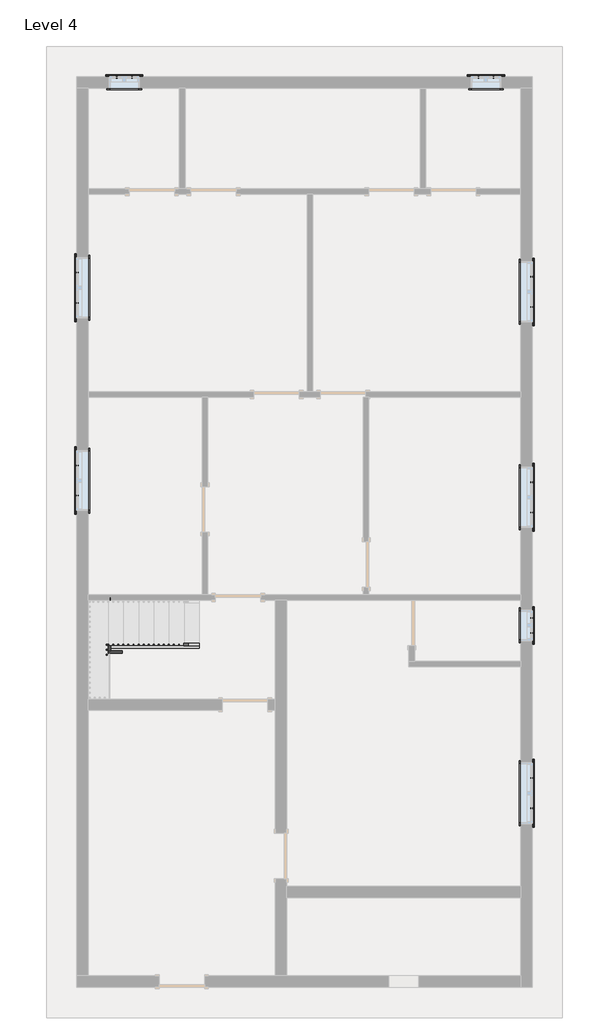
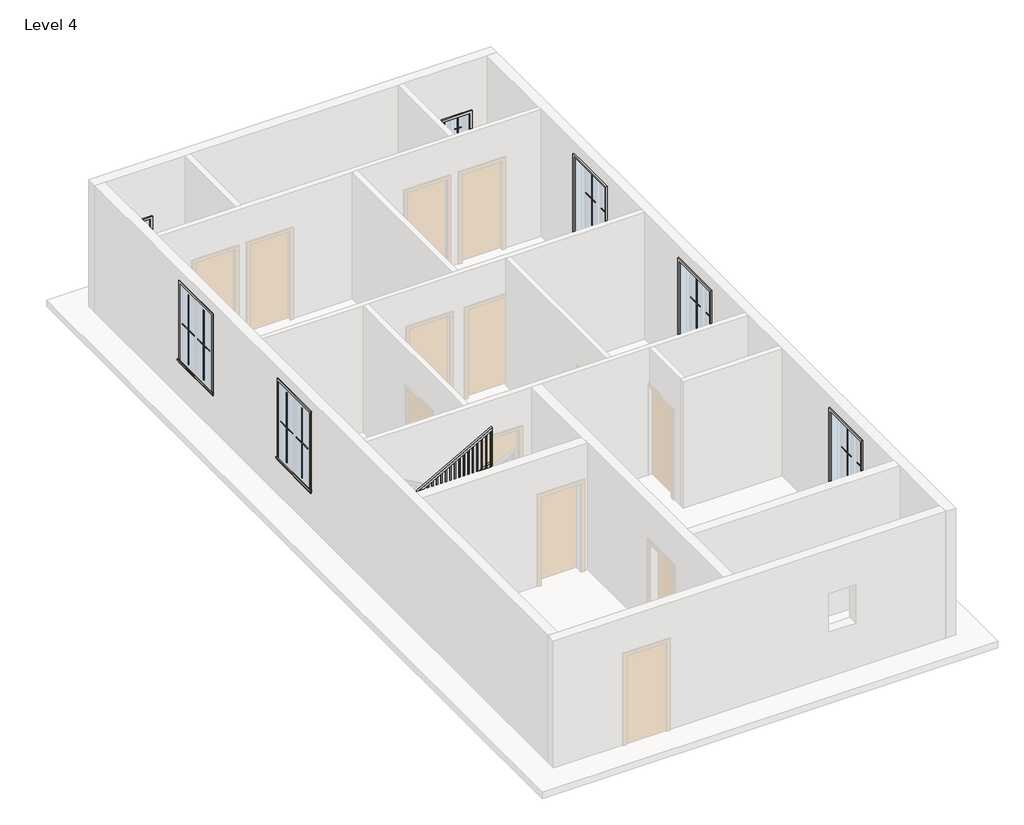
# One storey, part 3 of 3: 32 proxies, 6 members, 1 railing.
"""IFC4 building model written with IfcOpenShell, lengths in millimetres."""

from ifc_helpers import new_model, si_unit, frame, origin, place, context, project, spatial, polyline, outline, extrude, faceted_brep, transform, mapped, element, save
from components import muntin_pattern_2x2_muntin_pattern_2x2_2b4d9f72, muntin_pattern_2x2_muntin_pattern_2x2_ef995ed3, muntin_pattern_2x2_muntin_pattern_2x2_53152e2c, muntin_pattern_2x2_muntin_pattern_2x2_e8f3e573, trim_window_exterior_flat_with_sill_b7e4d11c, trim_window_exterior_flat_with_sill_a665a915, trim_window_interior_flat_picture_frame_936b8d2a, trim_window_interior_flat_picture_frame_d485c387

model = new_model("IFC4")

# Units and contexts
model_context = context("Model", 3, world=origin())
ifc_project = project(units=[si_unit("LENGTHUNIT", "METRE", prefix="MILLI")], contexts=[model_context])

# Site, building, storey
site = spatial("IfcSite", under=ifc_project)
building = spatial("IfcBuilding", under=site)
storey = spatial("IfcBuildingStorey", under=building, Name="Level 4", Elevation=9144.0)

# Proxies
placement = place(None, origin())
muntin_pattern_2x2_muntin_pattern_2x2_shape = muntin_pattern_2x2_muntin_pattern_2x2_2b4d9f72(model_context)
element("IfcBuildingElementProxy", 1, Name="Muntin Pattern_2x2 : Muntin Pattern_2x2", ObjectType="Muntin Pattern_2x2 : Muntin Pattern_2x2", at=placement, inside=storey, context=model_context, shape_type="MappedRepresentation", body=[
    mapped(muntin_pattern_2x2_muntin_pattern_2x2_shape, transform((1279.525, 5811.8375, 10128.25), x_axis=(0.0, 1.0, 0.0), y_axis=(-1.0, 0.0, 0.0), z_axis=(0.0, 0.0, 1.0))),
])
element("IfcBuildingElementProxy", 2, Name="Muntin Pattern_2x2 : Muntin Pattern_2x2", ObjectType="Muntin Pattern_2x2 : Muntin Pattern_2x2", at=placement, inside=storey, context=model_context, shape_type="MappedRepresentation", body=[
    mapped(muntin_pattern_2x2_muntin_pattern_2x2_shape, transform((1279.525, 9685.3375, 10128.25), x_axis=(0.0, 1.0, 0.0), y_axis=(-1.0, 0.0, 0.0), z_axis=(0.0, 0.0, 1.0))),
])
element("IfcBuildingElementProxy", 3, Name="Muntin Pattern_2x2 : Muntin Pattern_2x2", ObjectType="Muntin Pattern_2x2 : Muntin Pattern_2x2", at=placement, inside=storey, context=model_context, shape_type="MappedRepresentation", body=[
    mapped(muntin_pattern_2x2_muntin_pattern_2x2_shape, transform((10404.475, 10209.2125, 10128.25), x_axis=(0.0, -1.0, 0.0), y_axis=(1.0, 0.0, 0.0), z_axis=(0.0, 0.0, 1.0))),
])
element("IfcBuildingElementProxy", 4, Name="Muntin Pattern_2x2 : Muntin Pattern_2x2", ObjectType="Muntin Pattern_2x2 : Muntin Pattern_2x2", at=placement, inside=storey, context=model_context, shape_type="MappedRepresentation", body=[
    mapped(muntin_pattern_2x2_muntin_pattern_2x2_shape, transform((10404.475, 6081.7125, 10128.25), x_axis=(0.0, -1.0, 0.0), y_axis=(1.0, 0.0, 0.0), z_axis=(0.0, 0.0, 1.0))),
])
element("IfcBuildingElementProxy", 5, Name="Muntin Pattern_2x2 : Muntin Pattern_2x2", ObjectType="Muntin Pattern_2x2 : Muntin Pattern_2x2", at=placement, inside=storey, context=model_context, shape_type="MappedRepresentation", body=[
    mapped(muntin_pattern_2x2_muntin_pattern_2x2_shape, transform((10404.475, 138.1125, 10128.25), x_axis=(0.0, -1.0, 0.0), y_axis=(1.0, 0.0, 0.0), z_axis=(0.0, 0.0, 1.0))),
])
muntin_pattern_2x2_muntin_pattern_2x2_2_shape = muntin_pattern_2x2_muntin_pattern_2x2_ef995ed3(model_context)
element("IfcBuildingElementProxy", 6, Name="Muntin Pattern_2x2 : Muntin Pattern_2x2", ObjectType="Muntin Pattern_2x2 : Muntin Pattern_2x2", at=placement, inside=storey, context=model_context, shape_type="MappedRepresentation", body=[
    mapped(muntin_pattern_2x2_muntin_pattern_2x2_2_shape, transform((1279.525, 6418.2625, 10128.25), x_axis=(0.0, -1.0, 0.0), y_axis=(1.0, 0.0, 0.0), z_axis=(0.0, 0.0, 1.0))),
])
element("IfcBuildingElementProxy", 7, Name="Muntin Pattern_2x2 : Muntin Pattern_2x2", ObjectType="Muntin Pattern_2x2 : Muntin Pattern_2x2", at=placement, inside=storey, context=model_context, shape_type="MappedRepresentation", body=[
    mapped(muntin_pattern_2x2_muntin_pattern_2x2_2_shape, transform((1279.525, 10291.7625, 10128.25), x_axis=(0.0, -1.0, 0.0), y_axis=(1.0, 0.0, 0.0), z_axis=(0.0, 0.0, 1.0))),
])
element("IfcBuildingElementProxy", 8, Name="Muntin Pattern_2x2 : Muntin Pattern_2x2", ObjectType="Muntin Pattern_2x2 : Muntin Pattern_2x2", at=placement, inside=storey, context=model_context, shape_type="MappedRepresentation", body=[
    mapped(muntin_pattern_2x2_muntin_pattern_2x2_2_shape, transform((10404.475, 9602.7875, 10128.25), x_axis=(0.0, 1.0, 0.0), y_axis=(-1.0, 0.0, 0.0), z_axis=(0.0, 0.0, 1.0))),
])
element("IfcBuildingElementProxy", 9, Name="Muntin Pattern_2x2 : Muntin Pattern_2x2", ObjectType="Muntin Pattern_2x2 : Muntin Pattern_2x2", at=placement, inside=storey, context=model_context, shape_type="MappedRepresentation", body=[
    mapped(muntin_pattern_2x2_muntin_pattern_2x2_2_shape, transform((10404.475, 5475.2875, 10128.25), x_axis=(0.0, 1.0, 0.0), y_axis=(-1.0, 0.0, 0.0), z_axis=(0.0, 0.0, 1.0))),
])
element("IfcBuildingElementProxy", 10, Name="Muntin Pattern_2x2 : Muntin Pattern_2x2", ObjectType="Muntin Pattern_2x2 : Muntin Pattern_2x2", at=placement, inside=storey, context=model_context, shape_type="MappedRepresentation", body=[
    mapped(muntin_pattern_2x2_muntin_pattern_2x2_2_shape, transform((10404.475, -468.3125, 10128.25), x_axis=(0.0, 1.0, 0.0), y_axis=(-1.0, 0.0, 0.0), z_axis=(0.0, 0.0, 1.0))),
])
muntin_pattern_2x2_muntin_pattern_2x2_3_shape = muntin_pattern_2x2_muntin_pattern_2x2_53152e2c(model_context)
element("IfcBuildingElementProxy", 11, Name="Muntin Pattern_2x2 : Muntin Pattern_2x2", ObjectType="Muntin Pattern_2x2 : Muntin Pattern_2x2", at=placement, inside=storey, context=model_context, shape_type="MappedRepresentation", body=[
    mapped(muntin_pattern_2x2_muntin_pattern_2x2_3_shape, transform((10404.475, 3357.5625, 10128.25), x_axis=(0.0, -1.0, 0.0), y_axis=(1.0, 0.0, 0.0), z_axis=(0.0, 0.0, 1.0))),
])
element("IfcBuildingElementProxy", 12, Name="Muntin Pattern_2x2 : Muntin Pattern_2x2", ObjectType="Muntin Pattern_2x2 : Muntin Pattern_2x2", at=placement, inside=storey, context=model_context, shape_type="MappedRepresentation", body=[
    mapped(muntin_pattern_2x2_muntin_pattern_2x2_3_shape, transform((9336.0875, 14214.475, 10128.25), x_axis=(1.0, 0.0, 0.0), y_axis=(0.0, 1.0, 0.0), z_axis=(0.0, 0.0, 1.0))),
])
element("IfcBuildingElementProxy", 13, Name="Muntin Pattern_2x2 : Muntin Pattern_2x2", ObjectType="Muntin Pattern_2x2 : Muntin Pattern_2x2", at=placement, inside=storey, context=model_context, shape_type="MappedRepresentation", body=[
    mapped(muntin_pattern_2x2_muntin_pattern_2x2_3_shape, transform((2071.6875, 14214.475, 10128.25), x_axis=(1.0, 0.0, 0.0), y_axis=(0.0, 1.0, 0.0), z_axis=(0.0, 0.0, 1.0))),
])
muntin_pattern_2x2_muntin_pattern_2x2_4_shape = muntin_pattern_2x2_muntin_pattern_2x2_e8f3e573(model_context)
element("IfcBuildingElementProxy", 14, Name="Muntin Pattern_2x2 : Muntin Pattern_2x2", ObjectType="Muntin Pattern_2x2 : Muntin Pattern_2x2", at=placement, inside=storey, context=model_context, shape_type="MappedRepresentation", body=[
    mapped(muntin_pattern_2x2_muntin_pattern_2x2_4_shape, transform((10404.475, 3055.9375, 10128.25), x_axis=(0.0, 1.0, 0.0), y_axis=(-1.0, 0.0, 0.0), z_axis=(0.0, 0.0, 1.0))),
])
element("IfcBuildingElementProxy", 15, Name="Muntin Pattern_2x2 : Muntin Pattern_2x2", ObjectType="Muntin Pattern_2x2 : Muntin Pattern_2x2", at=placement, inside=storey, context=model_context, shape_type="MappedRepresentation", body=[
    mapped(muntin_pattern_2x2_muntin_pattern_2x2_4_shape, transform((9637.7125, 14214.475, 10128.25), x_axis=(-1.0, 0.0, 0.0), y_axis=(0.0, -1.0, 0.0), z_axis=(0.0, 0.0, 1.0))),
])
element("IfcBuildingElementProxy", 16, Name="Muntin Pattern_2x2 : Muntin Pattern_2x2", ObjectType="Muntin Pattern_2x2 : Muntin Pattern_2x2", at=placement, inside=storey, context=model_context, shape_type="MappedRepresentation", body=[
    mapped(muntin_pattern_2x2_muntin_pattern_2x2_4_shape, transform((2373.3125, 14214.475, 10128.25), x_axis=(-1.0, 0.0, 0.0), y_axis=(0.0, -1.0, 0.0), z_axis=(0.0, 0.0, 1.0))),
])
trim_window_exterior_flat_with_sill_shape = trim_window_exterior_flat_with_sill_b7e4d11c(model_context)
element("IfcBuildingElementProxy", 17, Name="Trim-Window-Exterior-Flat : with Sill", ObjectType="Trim-Window-Exterior-Flat : with Sill", at=placement, inside=storey, context=model_context, shape_type="MappedRepresentation", body=[
    mapped(trim_window_exterior_flat_with_sill_shape, transform((1270.0, 6115.05, 11887.2), x_axis=(0.0, -1.0, 0.0), y_axis=(0.0, 0.0, 1.0), z_axis=(-1.0, 0.0, 0.0))),
])
element("IfcBuildingElementProxy", 18, Name="Trim-Window-Exterior-Flat : with Sill", ObjectType="Trim-Window-Exterior-Flat : with Sill", at=placement, inside=storey, context=model_context, shape_type="MappedRepresentation", body=[
    mapped(trim_window_exterior_flat_with_sill_shape, transform((1270.0, 9988.55, 11887.2), x_axis=(0.0, -1.0, 0.0), y_axis=(0.0, 0.0, 1.0), z_axis=(-1.0, 0.0, 0.0))),
])
element("IfcBuildingElementProxy", 19, Name="Trim-Window-Exterior-Flat : with Sill", ObjectType="Trim-Window-Exterior-Flat : with Sill", at=placement, inside=storey, context=model_context, shape_type="MappedRepresentation", body=[
    mapped(trim_window_exterior_flat_with_sill_shape, transform((10414.0, 9906.0, 11887.2), x_axis=(0.0, 1.0, 0.0), y_axis=(0.0, 0.0, 1.0), z_axis=(1.0, 0.0, 0.0))),
])
element("IfcBuildingElementProxy", 20, Name="Trim-Window-Exterior-Flat : with Sill", ObjectType="Trim-Window-Exterior-Flat : with Sill", at=placement, inside=storey, context=model_context, shape_type="MappedRepresentation", body=[
    mapped(trim_window_exterior_flat_with_sill_shape, transform((10414.0, 5778.5, 11887.2), x_axis=(0.0, 1.0, 0.0), y_axis=(0.0, 0.0, 1.0), z_axis=(1.0, 0.0, 0.0))),
])
element("IfcBuildingElementProxy", 21, Name="Trim-Window-Exterior-Flat : with Sill", ObjectType="Trim-Window-Exterior-Flat : with Sill", at=placement, inside=storey, context=model_context, shape_type="MappedRepresentation", body=[
    mapped(trim_window_exterior_flat_with_sill_shape, transform((10414.0, -165.1, 11887.2), x_axis=(0.0, 1.0, 0.0), y_axis=(0.0, 0.0, 1.0), z_axis=(1.0, 0.0, 0.0))),
])
trim_window_exterior_flat_with_sill_2_shape = trim_window_exterior_flat_with_sill_a665a915(model_context)
element("IfcBuildingElementProxy", 22, Name="Trim-Window-Exterior-Flat : with Sill", ObjectType="Trim-Window-Exterior-Flat : with Sill", at=placement, inside=storey, context=model_context, shape_type="MappedRepresentation", body=[
    mapped(trim_window_exterior_flat_with_sill_2_shape, transform((10414.0, 3206.75, 10972.8), x_axis=(0.0, 1.0, 0.0), y_axis=(0.0, 0.0, 1.0), z_axis=(1.0, 0.0, 0.0))),
])
element("IfcBuildingElementProxy", 23, Name="Trim-Window-Exterior-Flat : with Sill", ObjectType="Trim-Window-Exterior-Flat : with Sill", at=placement, inside=storey, context=model_context, shape_type="MappedRepresentation", body=[
    mapped(trim_window_exterior_flat_with_sill_2_shape, transform((9486.9, 14224.0, 10972.8), x_axis=(-1.0, 0.0, 0.0), y_axis=(0.0, 0.0, 1.0), z_axis=(0.0, 1.0, 0.0))),
])
element("IfcBuildingElementProxy", 24, Name="Trim-Window-Exterior-Flat : with Sill", ObjectType="Trim-Window-Exterior-Flat : with Sill", at=placement, inside=storey, context=model_context, shape_type="MappedRepresentation", body=[
    mapped(trim_window_exterior_flat_with_sill_2_shape, transform((2222.5, 14224.0, 10972.8), x_axis=(-1.0, 0.0, 0.0), y_axis=(0.0, 0.0, 1.0), z_axis=(0.0, 1.0, 0.0))),
])
trim_window_interior_flat_picture_frame_shape = trim_window_interior_flat_picture_frame_936b8d2a(model_context)
element("IfcBuildingElementProxy", 25, Name="Trim-Window-Interior-Flat : Picture Frame", ObjectType="Trim-Window-Interior-Flat : Picture Frame", at=placement, inside=storey, context=model_context, shape_type="MappedRepresentation", body=[
    mapped(trim_window_interior_flat_picture_frame_shape, transform((1498.6, 6115.05, 11887.2), x_axis=(0.0, 1.0, 0.0), y_axis=(0.0, 0.0, 1.0), z_axis=(1.0, 0.0, 0.0))),
])
element("IfcBuildingElementProxy", 26, Name="Trim-Window-Interior-Flat : Picture Frame", ObjectType="Trim-Window-Interior-Flat : Picture Frame", at=placement, inside=storey, context=model_context, shape_type="MappedRepresentation", body=[
    mapped(trim_window_interior_flat_picture_frame_shape, transform((1498.6, 9988.55, 11887.2), x_axis=(0.0, 1.0, 0.0), y_axis=(0.0, 0.0, 1.0), z_axis=(1.0, 0.0, 0.0))),
])
element("IfcBuildingElementProxy", 27, Name="Trim-Window-Interior-Flat : Picture Frame", ObjectType="Trim-Window-Interior-Flat : Picture Frame", at=placement, inside=storey, context=model_context, shape_type="MappedRepresentation", body=[
    mapped(trim_window_interior_flat_picture_frame_shape, transform((10185.4, 9906.0, 11887.2), x_axis=(0.0, -1.0, 0.0), y_axis=(0.0, 0.0, 1.0), z_axis=(-1.0, 0.0, 0.0))),
])
element("IfcBuildingElementProxy", 28, Name="Trim-Window-Interior-Flat : Picture Frame", ObjectType="Trim-Window-Interior-Flat : Picture Frame", at=placement, inside=storey, context=model_context, shape_type="MappedRepresentation", body=[
    mapped(trim_window_interior_flat_picture_frame_shape, transform((10185.4, 5778.5, 11887.2), x_axis=(0.0, -1.0, 0.0), y_axis=(0.0, 0.0, 1.0), z_axis=(-1.0, 0.0, 0.0))),
])
element("IfcBuildingElementProxy", 29, Name="Trim-Window-Interior-Flat : Picture Frame", ObjectType="Trim-Window-Interior-Flat : Picture Frame", at=placement, inside=storey, context=model_context, shape_type="MappedRepresentation", body=[
    mapped(trim_window_interior_flat_picture_frame_shape, transform((10185.4, -165.1, 11887.2), x_axis=(0.0, -1.0, 0.0), y_axis=(0.0, 0.0, 1.0), z_axis=(-1.0, 0.0, 0.0))),
])
trim_window_interior_flat_picture_frame_2_shape = trim_window_interior_flat_picture_frame_d485c387(model_context)
element("IfcBuildingElementProxy", 30, Name="Trim-Window-Interior-Flat : Picture Frame", ObjectType="Trim-Window-Interior-Flat : Picture Frame", at=placement, inside=storey, context=model_context, shape_type="MappedRepresentation", body=[
    mapped(trim_window_interior_flat_picture_frame_2_shape, transform((10185.4, 3206.75, 10972.8), x_axis=(0.0, -1.0, 0.0), y_axis=(0.0, 0.0, 1.0), z_axis=(-1.0, 0.0, 0.0))),
])
element("IfcBuildingElementProxy", 31, Name="Trim-Window-Interior-Flat : Picture Frame", ObjectType="Trim-Window-Interior-Flat : Picture Frame", at=placement, inside=storey, context=model_context, shape_type="MappedRepresentation", body=[
    mapped(trim_window_interior_flat_picture_frame_2_shape, transform((9486.9, 13995.4, 10972.8), x_axis=(1.0, 0.0, 0.0), y_axis=(0.0, 0.0, 1.0), z_axis=(0.0, -1.0, 0.0))),
])
element("IfcBuildingElementProxy", 32, Name="Trim-Window-Interior-Flat : Picture Frame", ObjectType="Trim-Window-Interior-Flat : Picture Frame", at=placement, inside=storey, context=model_context, shape_type="MappedRepresentation", body=[
    mapped(trim_window_interior_flat_picture_frame_2_shape, transform((2222.5, 13995.4, 10972.8), x_axis=(1.0, 0.0, 0.0), y_axis=(0.0, 0.0, 1.0), z_axis=(0.0, -1.0, 0.0))),
])

# Members
element("IfcMember", 33, ObjectType="Stringer - 2\" Width", at=placement, inside=storey, context=model_context, shape_type="SweptSolid", body=[
    extrude(outline(polyline([(9144.0, 3727.9146873), (9351.5983948, 3727.9146873), (10339.3761726, 1949.9146873), (9990.6974984, 1949.9146873), (9144.0, 3473.9701845), (9144.0, 3727.9146873)])), frame((0.0, 2743.2, 0.0), z_axis=(0.0, 1.0, 0.0), x_axis=(0.0, 0.0, 1.0)), (0.0, 0.0, 1.0), 50.8),
])
element("IfcMember", 34, ObjectType="Stringer - 2\" Width", at=placement, inside=storey, context=model_context, shape_type="SweptSolid", body=[
    extrude(outline(polyline([(1899.1146873, 2794.0), (1949.9146873, 2794.0), (1949.9146873, 2692.4), (1899.1146873, 2692.4), (1899.1146873, 2794.0)])), frame((0.0, 0.0, 10100.7333333), z_axis=(0.0, 0.0, 1.0), x_axis=(1.0, 0.0, 0.0)), (0.0, 0.0, 1.0), 304.8),
])
element("IfcMember", 35, ObjectType="Stringer - 2\" Width", at=placement, inside=storey, context=model_context, shape_type="SweptSolid", body=[
    extrude(outline(polyline([(10536.9317281, 1899.1146873), (10188.253054, 1899.1146873), (11204.253054, 3727.9146873), (11552.9317281, 3727.9146873), (10536.9317281, 1899.1146873)])), frame((0.0, 2641.6, 0.0), z_axis=(0.0, 1.0, 0.0), x_axis=(0.0, 0.0, 1.0)), (0.0, 0.0, 1.0), 50.8),
])
element("IfcMember", 36, ObjectType="Stringer - 2\" Width", at=placement, inside=storey, context=model_context, shape_type="SweptSolid", body=[
    extrude(outline(polyline([(9144.0, 3727.9146873), (9351.5983948, 3727.9146873), (10405.5333333, 1830.8317979), (10405.5333333, 1498.6), (10241.4278803, 1498.6), (9144.0, 3473.9701845), (9144.0, 3727.9146873)])), frame((0.0, 3708.4, 0.0), z_axis=(0.0, 1.0, 0.0), x_axis=(0.0, 0.0, 1.0)), (0.0, 0.0, 1.0), 50.8),
])
element("IfcMember", 37, ObjectType="Stringer - 2\" Width", at=placement, inside=storey, context=model_context, shape_type="SweptSolid", body=[
    extrude(outline(polyline([(1447.8, 3759.2), (1498.6, 3759.2), (1498.6, 1727.2), (1447.8, 1727.2), (1447.8, 3759.2)])), frame((0.0, 0.0, 10100.7333333), z_axis=(0.0, 0.0, 1.0), x_axis=(1.0, 0.0, 0.0)), (0.0, 0.0, 1.0), 304.8),
])
element("IfcMember", 38, ObjectType="Stringer - 2\" Width", at=placement, inside=storey, context=model_context, shape_type="SweptSolid", body=[
    extrude(outline(polyline([(10286.2013463, 1447.8), (10100.7333333, 1447.8), (10100.7333333, 1741.5791901), (11204.253054, 3727.9146873), (11552.9317281, 3727.9146873), (10286.2013463, 1447.8)])), frame((0.0, 1676.4, 0.0), z_axis=(0.0, 1.0, 0.0), x_axis=(0.0, 0.0, 1.0)), (0.0, 0.0, 1.0), 50.8),
])

# Railing
element("IfcRailing", 39, ObjectType="Handrail - Rectangular", at=placement, inside=storey, context=model_context, shape_type="SolidModel", body=[
    faceted_brep([(3727.9146873, 2794.0, 10227.7333333), (3727.9146873, 2794.0, 10169.620221), (3727.9146873, 2844.8, 10169.620221), (3727.9146873, 2844.8, 10227.7333333), (1975.3146873, 2794.0, 11201.4), (1924.5146873, 2794.0, 11171.5091099), (1924.5146873, 2844.8, 11171.5091099), (1975.3146873, 2844.8, 11201.4), (1975.3146873, 2794.0, 11243.7333333), (1924.5146873, 2794.0, 11192.9333333), (1924.5146873, 2844.8, 11192.9333333), (1975.3146873, 2844.8, 11243.7333333), (1899.1146873, 2794.0, 11243.7333333), (1899.1146873, 2794.0, 11192.9333333), (1848.3146873, 2844.8, 11192.9333333), (1848.3146873, 2844.8, 11243.7333333), (1899.1146873, 2717.8, 11243.7333333), (1899.1146873, 2667.0, 11192.9333333), (1848.3146873, 2667.0, 11192.9333333), (1848.3146873, 2717.8, 11243.7333333), (1899.1146873, 2717.8, 11455.4), (1899.1146873, 2667.0, 11404.6), (1848.3146873, 2667.0, 11404.6), (1848.3146873, 2717.8, 11455.4), (1899.1146873, 2641.6, 11455.4), (1899.1146873, 2641.6, 11404.6), (1848.3146873, 2590.8, 11404.6), (1848.3146873, 2590.8, 11455.4), (1975.3146873, 2641.6, 11455.4), (1988.4782895, 2641.6, 11404.6), (1988.4782895, 2590.8, 11404.6), (1975.3146873, 2590.8, 11455.4), (3727.9146873, 2641.6, 12429.0666667), (3727.9146873, 2590.8, 12429.0666667), (3727.9146873, 2590.8, 12370.9535543), (3727.9146873, 2641.6, 12370.9535543)], [[[0, 1, 2, 3]], [[1, 0, 4, 5]], [[2, 1, 5, 6]], [[3, 2, 6, 7]], [[0, 3, 7, 4]], [[5, 4, 8, 9]], [[6, 5, 9, 10]], [[7, 6, 10, 11]], [[4, 7, 11, 8]], [[9, 8, 12, 13]], [[10, 9, 13, 14]], [[11, 10, 14, 15]], [[8, 11, 15, 12]], [[13, 12, 16, 17]], [[14, 13, 17, 18]], [[15, 14, 18, 19]], [[12, 15, 19, 16]], [[17, 16, 20, 21]], [[18, 17, 21, 22]], [[19, 18, 22, 23]], [[16, 19, 23, 20]], [[21, 20, 24, 25]], [[22, 21, 25, 26]], [[23, 22, 26, 27]], [[20, 23, 27, 24]], [[25, 24, 28, 29]], [[26, 25, 29, 30]], [[27, 26, 30, 31]], [[24, 27, 31, 28]], [[32, 33, 34, 35]], [[29, 28, 32, 35]], [[30, 29, 35, 34]], [[31, 30, 34, 33]], [[28, 31, 33, 32]]]),
    extrude(outline(polyline([(12351.5507765, 3692.9896873), (11345.3333333, 3692.9896873), (11345.3333333, 3712.0396873), (12362.1341099, 3712.0396873), (12351.5507765, 3692.9896873)])), frame((0.0, 2606.675, 0.0), z_axis=(0.0, 1.0, 0.0), x_axis=(0.0, 0.0, 1.0)), (0.0, 0.0, 1.0), 19.05),
    extrude(outline(polyline([(12295.1063321, 3591.3896873), (11345.3333333, 3591.3896873), (11345.3333333, 3610.4396873), (12305.6896654, 3610.4396873), (12295.1063321, 3591.3896873)])), frame((0.0, 2606.675, 0.0), z_axis=(0.0, 1.0, 0.0), x_axis=(0.0, 0.0, 1.0)), (0.0, 0.0, 1.0), 19.05),
    extrude(outline(polyline([(12238.6618876, 3489.7896873), (11345.3333333, 3489.7896873), (11345.3333333, 3508.8396873), (12249.245221, 3508.8396873), (12238.6618876, 3489.7896873)])), frame((0.0, 2606.675, 0.0), z_axis=(0.0, 1.0, 0.0), x_axis=(0.0, 0.0, 1.0)), (0.0, 0.0, 1.0), 19.05),
    extrude(outline(polyline([(12182.2174432, 3388.1896873), (11176.0, 3388.1896873), (11176.0, 3407.2396873), (12192.8007765, 3407.2396873), (12182.2174432, 3388.1896873)])), frame((0.0, 2606.675, 0.0), z_axis=(0.0, 1.0, 0.0), x_axis=(0.0, 0.0, 1.0)), (0.0, 0.0, 1.0), 19.05),
    extrude(outline(polyline([(12125.7729988, 3286.5896873), (11176.0, 3286.5896873), (11176.0, 3305.6396873), (12136.3563321, 3305.6396873), (12125.7729988, 3286.5896873)])), frame((0.0, 2606.675, 0.0), z_axis=(0.0, 1.0, 0.0), x_axis=(0.0, 0.0, 1.0)), (0.0, 0.0, 1.0), 19.05),
    extrude(outline(polyline([(12069.3285543, 3184.9896873), (11176.0, 3184.9896873), (11176.0, 3204.0396873), (12079.9118876, 3204.0396873), (12069.3285543, 3184.9896873)])), frame((0.0, 2606.675, 0.0), z_axis=(0.0, 1.0, 0.0), x_axis=(0.0, 0.0, 1.0)), (0.0, 0.0, 1.0), 19.05),
    extrude(outline(polyline([(12012.8841099, 3083.3896873), (11006.6666667, 3083.3896873), (11006.6666667, 3102.4396873), (12023.4674432, 3102.4396873), (12012.8841099, 3083.3896873)])), frame((0.0, 2606.675, 0.0), z_axis=(0.0, 1.0, 0.0), x_axis=(0.0, 0.0, 1.0)), (0.0, 0.0, 1.0), 19.05),
    extrude(outline(polyline([(11956.4396654, 2981.7896873), (11006.6666667, 2981.7896873), (11006.6666667, 3000.8396873), (11967.0229988, 3000.8396873), (11956.4396654, 2981.7896873)])), frame((0.0, 2606.675, 0.0), z_axis=(0.0, 1.0, 0.0), x_axis=(0.0, 0.0, 1.0)), (0.0, 0.0, 1.0), 19.05),
    extrude(outline(polyline([(11899.995221, 2880.1896873), (11006.6666667, 2880.1896873), (11006.6666667, 2899.2396873), (11910.5785543, 2899.2396873), (11899.995221, 2880.1896873)])), frame((0.0, 2606.675, 0.0), z_axis=(0.0, 1.0, 0.0), x_axis=(0.0, 0.0, 1.0)), (0.0, 0.0, 1.0), 19.05),
    extrude(outline(polyline([(11843.5507765, 2778.5896873), (10837.3333333, 2778.5896873), (10837.3333333, 2797.6396873), (11854.1341099, 2797.6396873), (11843.5507765, 2778.5896873)])), frame((0.0, 2606.675, 0.0), z_axis=(0.0, 1.0, 0.0), x_axis=(0.0, 0.0, 1.0)), (0.0, 0.0, 1.0), 19.05),
    extrude(outline(polyline([(11787.1063321, 2676.9896873), (10837.3333333, 2676.9896873), (10837.3333333, 2696.0396873), (11797.6896654, 2696.0396873), (11787.1063321, 2676.9896873)])), frame((0.0, 2606.675, 0.0), z_axis=(0.0, 1.0, 0.0), x_axis=(0.0, 0.0, 1.0)), (0.0, 0.0, 1.0), 19.05),
    extrude(outline(polyline([(11730.6618876, 2575.3896873), (10837.3333333, 2575.3896873), (10837.3333333, 2594.4396873), (11741.245221, 2594.4396873), (11730.6618876, 2575.3896873)])), frame((0.0, 2606.675, 0.0), z_axis=(0.0, 1.0, 0.0), x_axis=(0.0, 0.0, 1.0)), (0.0, 0.0, 1.0), 19.05),
    extrude(outline(polyline([(11674.2174432, 2473.7896873), (10668.0, 2473.7896873), (10668.0, 2492.8396873), (11684.8007765, 2492.8396873), (11674.2174432, 2473.7896873)])), frame((0.0, 2606.675, 0.0), z_axis=(0.0, 1.0, 0.0), x_axis=(0.0, 0.0, 1.0)), (0.0, 0.0, 1.0), 19.05),
    extrude(outline(polyline([(11617.7729988, 2372.1896873), (10668.0, 2372.1896873), (10668.0, 2391.2396873), (11628.3563321, 2391.2396873), (11617.7729988, 2372.1896873)])), frame((0.0, 2606.675, 0.0), z_axis=(0.0, 1.0, 0.0), x_axis=(0.0, 0.0, 1.0)), (0.0, 0.0, 1.0), 19.05),
    extrude(outline(polyline([(11561.3285543, 2270.5896873), (10668.0, 2270.5896873), (10668.0, 2289.6396873), (11571.9118876, 2289.6396873), (11561.3285543, 2270.5896873)])), frame((0.0, 2606.675, 0.0), z_axis=(0.0, 1.0, 0.0), x_axis=(0.0, 0.0, 1.0)), (0.0, 0.0, 1.0), 19.05),
    extrude(outline(polyline([(11504.8841099, 2168.9896873), (10498.6666667, 2168.9896873), (10498.6666667, 2188.0396873), (11515.4674432, 2188.0396873), (11504.8841099, 2168.9896873)])), frame((0.0, 2606.675, 0.0), z_axis=(0.0, 1.0, 0.0), x_axis=(0.0, 0.0, 1.0)), (0.0, 0.0, 1.0), 19.05),
    extrude(outline(polyline([(11448.4396654, 2067.3896873), (10498.6666667, 2067.3896873), (10498.6666667, 2086.4396873), (11459.0229988, 2086.4396873), (11448.4396654, 2067.3896873)])), frame((0.0, 2606.675, 0.0), z_axis=(0.0, 1.0, 0.0), x_axis=(0.0, 0.0, 1.0)), (0.0, 0.0, 1.0), 19.05),
    extrude(outline(polyline([(11391.995221, 1965.7896873), (10498.6666667, 1965.7896873), (10498.6666667, 1984.8396873), (11402.5785543, 1984.8396873), (11391.995221, 1965.7896873)])), frame((0.0, 2606.675, 0.0), z_axis=(0.0, 1.0, 0.0), x_axis=(0.0, 0.0, 1.0)), (0.0, 0.0, 1.0), 19.05),
    extrude(outline(polyline([(1883.2396873, 2727.325), (1883.2396873, 2708.275), (1864.1896873, 2708.275), (1864.1896873, 2727.325), (1883.2396873, 2727.325)])), frame((0.0, 0.0, 10329.3333333), z_axis=(0.0, 0.0, 1.0), x_axis=(1.0, 0.0, 0.0)), (0.0, 0.0, 1.0), 863.6),
    extrude(outline(polyline([(1908.6396873, 2809.875), (1889.5896873, 2809.875), (1889.5896873, 2828.925), (1908.6396873, 2828.925), (1908.6396873, 2809.875)])), frame((0.0, 0.0, 10329.3333333), z_axis=(0.0, 0.0, 1.0), x_axis=(1.0, 0.0, 0.0)), (0.0, 0.0, 1.0), 863.6),
    extrude(outline(polyline([(11134.4674432, 1991.1896873), (10160.0, 1991.1896873), (10160.0, 2010.2396873), (11123.8841099, 2010.2396873), (11134.4674432, 1991.1896873)])), frame((0.0, 2809.875, 0.0), z_axis=(0.0, 1.0, 0.0), x_axis=(0.0, 0.0, 1.0)), (0.0, 0.0, 1.0), 19.05),
    extrude(outline(polyline([(11078.0229988, 2092.7896873), (10160.0, 2092.7896873), (10160.0, 2111.8396873), (11067.4396654, 2111.8396873), (11078.0229988, 2092.7896873)])), frame((0.0, 2809.875, 0.0), z_axis=(0.0, 1.0, 0.0), x_axis=(0.0, 0.0, 1.0)), (0.0, 0.0, 1.0), 19.05),
    extrude(outline(polyline([(11021.5785543, 2194.3896873), (10160.0, 2194.3896873), (10160.0, 2213.4396873), (11010.995221, 2213.4396873), (11021.5785543, 2194.3896873)])), frame((0.0, 2809.875, 0.0), z_axis=(0.0, 1.0, 0.0), x_axis=(0.0, 0.0, 1.0)), (0.0, 0.0, 1.0), 19.05),
    extrude(outline(polyline([(10965.1341099, 2295.9896873), (9990.6666667, 2295.9896873), (9990.6666667, 2315.0396873), (10954.5507765, 2315.0396873), (10965.1341099, 2295.9896873)])), frame((0.0, 2809.875, 0.0), z_axis=(0.0, 1.0, 0.0), x_axis=(0.0, 0.0, 1.0)), (0.0, 0.0, 1.0), 19.05),
    extrude(outline(polyline([(10908.6896654, 2397.5896873), (9990.6666667, 2397.5896873), (9990.6666667, 2416.6396873), (10898.1063321, 2416.6396873), (10908.6896654, 2397.5896873)])), frame((0.0, 2809.875, 0.0), z_axis=(0.0, 1.0, 0.0), x_axis=(0.0, 0.0, 1.0)), (0.0, 0.0, 1.0), 19.05),
    extrude(outline(polyline([(10852.245221, 2499.1896873), (9990.6666667, 2499.1896873), (9990.6666667, 2518.2396873), (10841.6618876, 2518.2396873), (10852.245221, 2499.1896873)])), frame((0.0, 2809.875, 0.0), z_axis=(0.0, 1.0, 0.0), x_axis=(0.0, 0.0, 1.0)), (0.0, 0.0, 1.0), 19.05),
    extrude(outline(polyline([(10795.8007765, 2600.7896873), (9821.3333333, 2600.7896873), (9821.3333333, 2619.8396873), (10785.2174432, 2619.8396873), (10795.8007765, 2600.7896873)])), frame((0.0, 2809.875, 0.0), z_axis=(0.0, 1.0, 0.0), x_axis=(0.0, 0.0, 1.0)), (0.0, 0.0, 1.0), 19.05),
    extrude(outline(polyline([(10739.3563321, 2702.3896873), (9821.3333333, 2702.3896873), (9821.3333333, 2721.4396873), (10728.7729988, 2721.4396873), (10739.3563321, 2702.3896873)])), frame((0.0, 2809.875, 0.0), z_axis=(0.0, 1.0, 0.0), x_axis=(0.0, 0.0, 1.0)), (0.0, 0.0, 1.0), 19.05),
    extrude(outline(polyline([(10682.9118876, 2803.9896873), (9821.3333333, 2803.9896873), (9821.3333333, 2823.0396873), (10672.3285543, 2823.0396873), (10682.9118876, 2803.9896873)])), frame((0.0, 2809.875, 0.0), z_axis=(0.0, 1.0, 0.0), x_axis=(0.0, 0.0, 1.0)), (0.0, 0.0, 1.0), 19.05),
    extrude(outline(polyline([(10626.4674432, 2905.5896873), (9652.0, 2905.5896873), (9652.0, 2924.6396873), (10615.8841099, 2924.6396873), (10626.4674432, 2905.5896873)])), frame((0.0, 2809.875, 0.0), z_axis=(0.0, 1.0, 0.0), x_axis=(0.0, 0.0, 1.0)), (0.0, 0.0, 1.0), 19.05),
    extrude(outline(polyline([(10570.0229988, 3007.1896873), (9652.0, 3007.1896873), (9652.0, 3026.2396873), (10559.4396654, 3026.2396873), (10570.0229988, 3007.1896873)])), frame((0.0, 2809.875, 0.0), z_axis=(0.0, 1.0, 0.0), x_axis=(0.0, 0.0, 1.0)), (0.0, 0.0, 1.0), 19.05),
    extrude(outline(polyline([(10513.5785543, 3108.7896873), (9652.0, 3108.7896873), (9652.0, 3127.8396873), (10502.995221, 3127.8396873), (10513.5785543, 3108.7896873)])), frame((0.0, 2809.875, 0.0), z_axis=(0.0, 1.0, 0.0), x_axis=(0.0, 0.0, 1.0)), (0.0, 0.0, 1.0), 19.05),
    extrude(outline(polyline([(10457.1341099, 3210.3896873), (9482.6666667, 3210.3896873), (9482.6666667, 3229.4396873), (10446.5507765, 3229.4396873), (10457.1341099, 3210.3896873)])), frame((0.0, 2809.875, 0.0), z_axis=(0.0, 1.0, 0.0), x_axis=(0.0, 0.0, 1.0)), (0.0, 0.0, 1.0), 19.05),
    extrude(outline(polyline([(10400.6896654, 3311.9896873), (9482.6666667, 3311.9896873), (9482.6666667, 3331.0396873), (10390.1063321, 3331.0396873), (10400.6896654, 3311.9896873)])), frame((0.0, 2809.875, 0.0), z_axis=(0.0, 1.0, 0.0), x_axis=(0.0, 0.0, 1.0)), (0.0, 0.0, 1.0), 19.05),
    extrude(outline(polyline([(10344.245221, 3413.5896873), (9482.6666667, 3413.5896873), (9482.6666667, 3432.6396873), (10333.6618876, 3432.6396873), (10344.245221, 3413.5896873)])), frame((0.0, 2809.875, 0.0), z_axis=(0.0, 1.0, 0.0), x_axis=(0.0, 0.0, 1.0)), (0.0, 0.0, 1.0), 19.05),
    extrude(outline(polyline([(10287.8007765, 3515.1896873), (9313.3333333, 3515.1896873), (9313.3333333, 3534.2396873), (10277.2174432, 3534.2396873), (10287.8007765, 3515.1896873)])), frame((0.0, 2809.875, 0.0), z_axis=(0.0, 1.0, 0.0), x_axis=(0.0, 0.0, 1.0)), (0.0, 0.0, 1.0), 19.05),
    extrude(outline(polyline([(10231.3563321, 3616.7896873), (9313.3333333, 3616.7896873), (9313.3333333, 3635.8396873), (10220.7729988, 3635.8396873), (10231.3563321, 3616.7896873)])), frame((0.0, 2809.875, 0.0), z_axis=(0.0, 1.0, 0.0), x_axis=(0.0, 0.0, 1.0)), (0.0, 0.0, 1.0), 19.05),
    extrude(outline(polyline([(1883.2396873, 2625.725), (1883.2396873, 2606.675), (1864.1896873, 2606.675), (1864.1896873, 2625.725), (1883.2396873, 2625.725)])), frame((0.0, 0.0, 10329.3333333), z_axis=(0.0, 0.0, 1.0), x_axis=(1.0, 0.0, 0.0)), (0.0, 0.0, 1.0), 1075.2666667),
    extrude(outline(polyline([(1883.2396873, 2809.875), (1864.1896873, 2809.875), (1864.1896873, 2828.925), (1883.2396873, 2828.925), (1883.2396873, 2809.875)])), frame((0.0, 0.0, 10329.3333333), z_axis=(0.0, 0.0, 1.0), x_axis=(1.0, 0.0, 0.0)), (0.0, 0.0, 1.0), 863.6),
    extrude(outline(polyline([(12360.370221, 3708.8646873), (11345.3333333, 3708.8646873), (11345.3333333, 3727.9146873), (12370.9535543, 3727.9146873), (12360.370221, 3708.8646873)])), frame((0.0, 2606.675, 0.0), z_axis=(0.0, 1.0, 0.0), x_axis=(0.0, 0.0, 1.0)), (0.0, 0.0, 1.0), 19.05),
    extrude(outline(polyline([(10180.2035543, 3708.8646873), (9313.3333333, 3708.8646873), (9313.3333333, 3727.9146873), (10169.620221, 3727.9146873), (10180.2035543, 3708.8646873)])), frame((0.0, 2809.875, 0.0), z_axis=(0.0, 1.0, 0.0), x_axis=(0.0, 0.0, 1.0)), (0.0, 0.0, 1.0), 19.05),
])

save(model, "model.ifc")

# Revit data of these elements
# Type "Muntin Pattern_2x2 : Muntin Pattern_2x2"
#   Width [instance default] = 4' - 0"
#   Thickness = 0' - 0 1/2"
#   Height [instance default] = 4' - 0"
#   Distance = 0' - 0 3/4"
#   Interior Material [instance default] = none
#   Exterior Material [instance default] = none
#   Default Elevation = 0
# Type "Trim-Window-Exterior-Flat : with Sill"
#   Trim Width = 0' - 2 1/4"
#   Trim Thickness_Picture Frame = 0' - 1 1/4"
#   Trim Thickness_with Sill = 0' - 0 3/4"
#   Sill Thickness = 0' - 1 1/4"
#   Opening Width [instance default] = 2' - 0"
#   Opening Height [instance default] = 3' - 0"
#   Default Elevation = 4' - 0"
#   Sill = yes
#   Picture Frame = no
#   Trim Material [instance default] = none
# Type "Trim-Window-Interior-Flat : Picture Frame"
#   Trim Thickness_Picture Frame = 0' - 1 1/4"
#   Trim Width = 0' - 2 1/4"
#   Trim Thickness_with Sill = 0' - 0 3/4"
#   Sill Thickness = 0' - 1 1/4"
#   Opening Width [instance default] = 2' - 0"
#   Opening Height [instance default] = 3' - 0"
#   Default Elevation = 4' - 0"
#   Sill = no
#   Picture Frame = yes
#   Trim Material [instance default] = none
# Type "Handrail - Rectangular"
#   Assembly Code = "C2010400"
#   built-in parameter 1008612 = 0.0416667 (stored number, unit not read)
#   built-in parameter 1008611 = 0.0416667 (stored number, unit not read)
#   built-in parameter 1008609 = 0.333333 (stored number, unit not read)
#   built-in parameter 1008604 = 0.166667 (stored number, unit not read)
#   built-in parameter 1008603 = 0.166667 (stored number, unit not read)
#   Railing Height = 3' - 0"
#   built-in parameter 1008630 = 2
#   built-in parameter 1008610 = 2
#   built-in parameter 1008618 = Baluster - Square : 3/4"
# Elements 1, 2, 3, 4, 5, 6, 7, 8, 9, 10 (IfcBuildingElementProxy, "Muntin Pattern_2x2 : Muntin Pattern_2x2")
#   Width = 1' - 6 5/8"
#   Height = 5' - 6 1/2"
#   Interior Material = Wood - Stained
#   Exterior Material = Clad - White
#   Phase Created = New Construction
#   Materials on its faces: "Clad - White", "Wood - Stained"
# Elements 11, 12, 13, 14, 15, 16 (IfcBuildingElementProxy, "Muntin Pattern_2x2 : Muntin Pattern_2x2")
#   Width = 0' - 6 5/8"
#   Height = 2' - 6 1/2"
#   Interior Material = Wood - Stained
#   Exterior Material = Clad - White
#   Phase Created = New Construction
#   Materials on its faces: "Clad - White", "Wood - Stained"
# Elements 17, 18, 19, 20, 21 (IfcBuildingElementProxy, "Trim-Window-Exterior-Flat : with Sill")
#   Opening Width = 4' - 0"
#   Opening Height = 6' - 0"
#   Trim Material = Clad - White
#   Phase Created = New Construction
#   Materials on its faces: "Clad - White"
# Elements 22, 23, 24 (IfcBuildingElementProxy, "Trim-Window-Exterior-Flat : with Sill")
#   Opening Width = 2' - 0"
#   Opening Height = 3' - 0"
#   Trim Material = Clad - White
#   Phase Created = New Construction
#   Materials on its faces: "Clad - White"
# Elements 25, 26, 27, 28, 29 (IfcBuildingElementProxy, "Trim-Window-Interior-Flat : Picture Frame")
#   Opening Width = 4' - 0"
#   Opening Height = 6' - 0"
#   Trim Material = Wood - Stained
#   Phase Created = New Construction
#   Materials on its faces: "Wood - Stained"
# Elements 30, 31, 32 (IfcBuildingElementProxy, "Trim-Window-Interior-Flat : Picture Frame")
#   Opening Width = 2' - 0"
#   Opening Height = 3' - 0"
#   Trim Material = Wood - Stained
#   Phase Created = New Construction
#   Materials on its faces: "Wood - Stained"
# Elements 33, 34, 35, 36, 37, 38 (IfcMember, "Stringer - 2\" Width")
#   Phase Created = New Construction
# Element 39 (IfcRailing, "Handrail - Rectangular")
#   Phase Created = New Construction
# Materials
#   "Clad - White": class "Wood", colour RGB 242 242 238, transparency 0, Cost = 0
#   "Wood - Stained": class "Wood", colour RGB 224 178 126, transparency 0, Cost = 0
